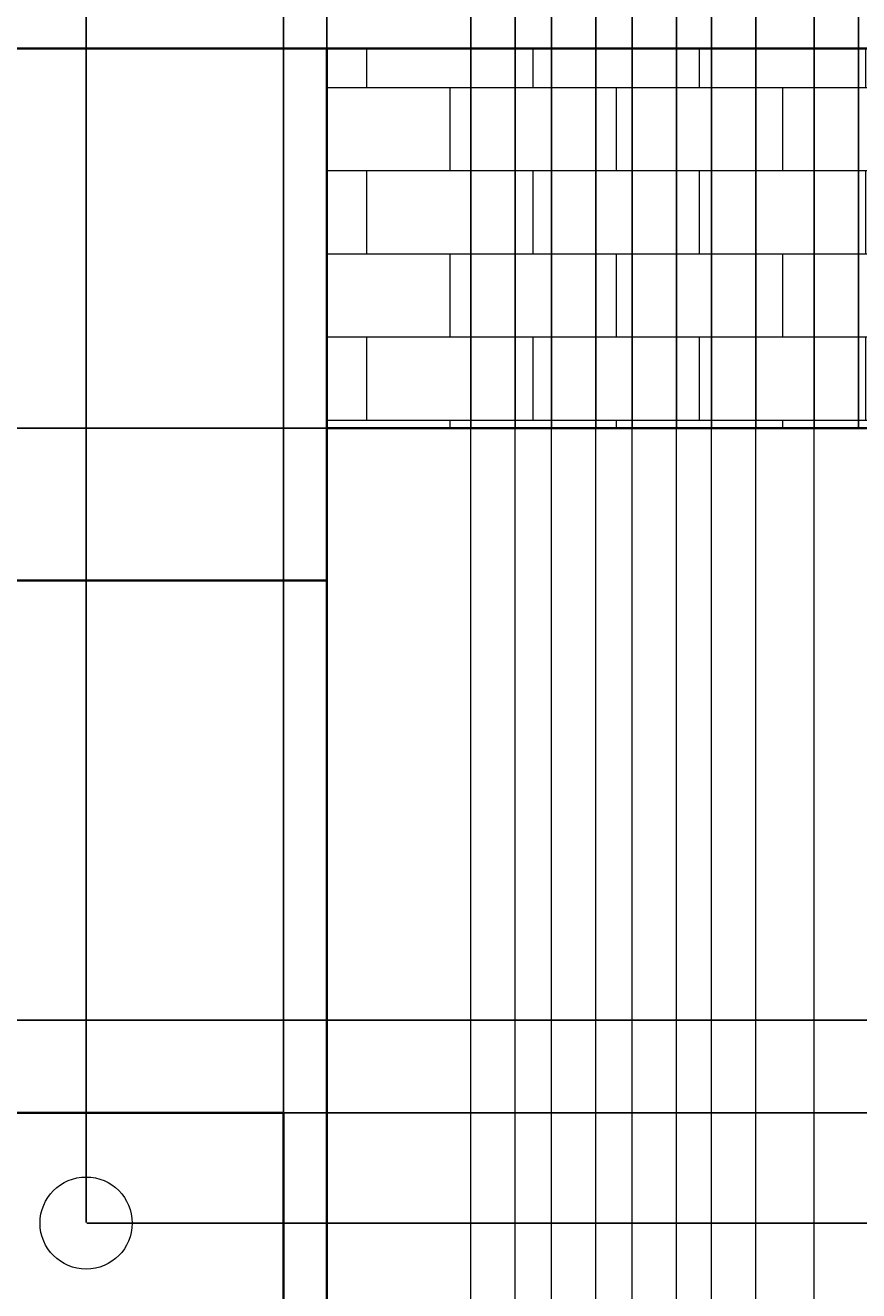
# Model space of a CAD drawing. Units: inches. Extents: x -13 to 809, y 112 to 656.
# Tile 34 of 55: x 314 to 389, y 446 to 561. Entities that reach past the tile are written whole.
import ezdxf

# ---------------------------------------------------------------- set-up
doc = ezdxf.new("R2010")
doc.units = ezdxf.units.IN
doc.header["$MEASUREMENT"] = 0
for name, color, linetype, lineweight in [('A-ANNO-DIMS', 2, 'Continuous', 18), ('A-ELEV', 7, 'Continuous', 35), ('A-ELEV-OTLN', 7, 'Continuous', 18), ('A-ELEV-PATT', 8, 'Continuous', 13)]:
    doc.layers.add(name, color=color, linetype=linetype, lineweight=lineweight)
doc.styles.get("Standard").update_dxf_attribs({"font": 'arial.ttf'})
doc.dimstyles.get("Standard").update_dxf_attribs({"dimtxt": 0.625, "dimasz": 0.18, "dimexe": 0.18, "dimexo": 0.0625, "dimgap": 0.09, "dimtad": 0, "dimtih": 1, "dimtoh": 1, "dimdec": 4, "dimzin": 0, "dimdsep": 46, "dimlunit": 4, "dimtxsty": 'Standard', "dimcen": 0.09, "dimadec": 0, "dimazin": 0, "dimtfac": 1, "dimtdec": 4, "dimtofl": 0, "dimtmove": 0, "dimatfit": 3, "dimfxl": 1, "dimtolj": 1, "dimtzin": 0, "dimarcsym": 0})

# ---------------------------------------------------------------- blocks, each defined once
blk = doc.blocks.new('*D25')
at = {"layer": 'A-ANNO-DIMS', "color": 0, "lineweight": -2, "transparency": 16777216}
for p, q in [((311.7, 617.43), (311.7, 655.96)), ((311.88, 655.78), (325.46, 655.78)), ((341.23, 655.78), (327.64, 655.78)), ((341.41, 524.34), (341.41, 655.96))]:
    blk.add_line(p, q, dxfattribs=at)
at = {"layer": 'A-ANNO-DIMS', "color": 0, "transparency": 16777216}
for points in [[(311.88, 655.81), (311.88, 655.75), (311.7, 655.78)], [(341.23, 655.81), (341.23, 655.75), (341.41, 655.78)]]:
    blk.add_solid(points, dxfattribs=at)
at = {"layer": 'Defpoints', "color": 0, "transparency": 16777216}
for p in [(341.41, 655.78), (311.7, 617.37), (341.41, 524.28)]:
    blk.add_point(p, dxfattribs=at)
at = {"layer": 'A-ANNO-DIMS', "color": 0, "transparency": 16777216, "insert": (326.55, 655.78), "char_height": 0.625, "attachment_point": 5}
blk.add_mtext('\\A1;29.71', dxfattribs=at)
blk = doc.blocks.new('*D26')
at = {"layer": 'A-ANNO-DIMS', "color": 0, "lineweight": -2, "transparency": 16777216}
for p, q in [((341.41, 524.34), (341.41, 655.96)), ((341.59, 655.78), (405.14, 655.78)), ((470.92, 655.78), (407.37, 655.78)), ((471.1, 470.94), (471.1, 655.96))]:
    blk.add_line(p, q, dxfattribs=at)
at = {"layer": 'A-ANNO-DIMS', "color": 0, "transparency": 16777216}
for points in [[(341.59, 655.81), (341.59, 655.75), (341.41, 655.78)], [(470.92, 655.81), (470.92, 655.75), (471.1, 655.78)]]:
    blk.add_solid(points, dxfattribs=at)
at = {"layer": 'Defpoints', "color": 0, "transparency": 16777216}
for p in [(471.1, 655.78), (341.41, 524.28), (471.1, 470.88)]:
    blk.add_point(p, dxfattribs=at)
at = {"layer": 'A-ANNO-DIMS', "color": 0, "transparency": 16777216, "insert": (406.25, 655.78), "char_height": 0.625, "attachment_point": 5}
blk.add_mtext('\\A1;129.7', dxfattribs=at)
blk = doc.blocks.new('*D39')
at = {"layer": 'A-ANNO-DIMS', "color": 0, "lineweight": -2, "transparency": 16777216}
for p, q in [((341.34, 524.28), (-12.1, 524.28)), ((-11.92, 524.1), (-11.92, 406.78)), ((-11.92, 288.63), (-11.92, 405.96)), ((341.34, 288.45), (-12.1, 288.45))]:
    blk.add_line(p, q, dxfattribs=at)
at = {"layer": 'A-ANNO-DIMS', "color": 0, "transparency": 16777216}
for points in [[(-11.95, 524.1), (-11.89, 524.1), (-11.92, 524.28)], [(-11.95, 288.63), (-11.89, 288.63), (-11.92, 288.45)]]:
    blk.add_solid(points, dxfattribs=at)
at = {"layer": 'Defpoints', "color": 0, "transparency": 16777216}
for p in [(-11.92, 524.28), (341.41, 524.28), (341.41, 288.45)]:
    blk.add_point(p, dxfattribs=at)
at = {"layer": 'A-ANNO-DIMS', "color": 0, "transparency": 16777216, "insert": (-11.92, 406.37), "char_height": 0.625, "attachment_point": 5}
blk.add_mtext('\\A1;235.83', dxfattribs=at)
blk = doc.blocks.new('*D43')
at = {"layer": 'A-ANNO-DIMS', "color": 0, "lineweight": -2, "transparency": 16777216}
for p, q in [((471.04, 470.88), (-12.1, 470.88)), ((-11.92, 470.7), (-11.92, 443.28)), ((-11.92, 415.04), (-11.92, 442.46)), ((471.04, 414.86), (-12.1, 414.86))]:
    blk.add_line(p, q, dxfattribs=at)
at = {"layer": 'A-ANNO-DIMS', "color": 0, "transparency": 16777216}
for points in [[(-11.95, 470.7), (-11.89, 470.7), (-11.92, 470.88)], [(-11.95, 415.04), (-11.89, 415.04), (-11.92, 414.86)]]:
    blk.add_solid(points, dxfattribs=at)
at = {"layer": 'Defpoints', "color": 0, "transparency": 16777216}
for p in [(-11.92, 470.88), (471.1, 470.88), (471.1, 414.86)]:
    blk.add_point(p, dxfattribs=at)
at = {"layer": 'A-ANNO-DIMS', "color": 0, "transparency": 16777216, "insert": (-11.92, 442.87), "char_height": 0.625, "attachment_point": 5}
blk.add_mtext('\\A1;56.02', dxfattribs=at)
blk = doc.blocks.new('*D53')
at = {"layer": 'A-ANNO-DIMS', "color": 0, "lineweight": -2, "transparency": 16777216}
for p, q in [((341.41, 524.34), (341.41, 655.96)), ((341.59, 655.78), (346.6, 655.78)), ((354.21, 655.78), (349.2, 655.78)), ((354.39, 524.34), (354.39, 655.96))]:
    blk.add_line(p, q, dxfattribs=at)
at = {"layer": 'A-ANNO-DIMS', "color": 0, "transparency": 16777216}
for points in [[(341.59, 655.81), (341.59, 655.75), (341.41, 655.78)], [(354.21, 655.81), (354.21, 655.75), (354.39, 655.78)]]:
    blk.add_solid(points, dxfattribs=at)
at = {"layer": 'Defpoints', "color": 0, "transparency": 16777216}
for p in [(354.39, 655.78), (341.41, 524.28), (354.39, 524.28)]:
    blk.add_point(p, dxfattribs=at)
at = {"layer": 'A-ANNO-DIMS', "color": 0, "transparency": 16777216, "insert": (347.9, 655.78), "char_height": 0.625, "attachment_point": 5}
blk.add_mtext('\\A1;12.981', dxfattribs=at)
blk = doc.blocks.new('*D54')
at = {"layer": 'A-ANNO-DIMS', "color": 0, "lineweight": -2, "transparency": 16777216}
for p, q in [((354.39, 524.34), (354.39, 655.96)), ((354.57, 655.78), (356.08, 655.78)), ((358.21, 655.78), (356.69, 655.78)), ((358.39, 524.34), (358.39, 655.96))]:
    blk.add_line(p, q, dxfattribs=at)
at = {"layer": 'A-ANNO-DIMS', "color": 0, "transparency": 16777216}
for points in [[(354.57, 655.81), (354.57, 655.75), (354.39, 655.78)], [(358.21, 655.81), (358.21, 655.75), (358.39, 655.78)]]:
    blk.add_solid(points, dxfattribs=at)
at = {"layer": 'Defpoints', "color": 0, "transparency": 16777216}
for p in [(358.39, 655.78), (354.39, 524.28), (358.39, 524.28)]:
    blk.add_point(p, dxfattribs=at)
at = {"layer": 'A-ANNO-DIMS', "color": 0, "transparency": 16777216, "insert": (356.39, 655.78), "char_height": 0.625, "attachment_point": 5}
blk.add_mtext('\\A1;4', dxfattribs=at)
blk = doc.blocks.new('*D55')
at = {"layer": 'A-ANNO-DIMS', "color": 0, "lineweight": -2, "transparency": 16777216}
for p, q in [((358.39, 524.34), (358.39, 655.96)), ((358.57, 655.78), (358.88, 655.78)), ((361.48, 655.78), (361.17, 655.78)), ((361.66, 524.34), (361.66, 655.96))]:
    blk.add_line(p, q, dxfattribs=at)
at = {"layer": 'A-ANNO-DIMS', "color": 0, "transparency": 16777216}
for points in [[(358.57, 655.81), (358.57, 655.75), (358.39, 655.78)], [(361.48, 655.81), (361.48, 655.75), (361.66, 655.78)]]:
    blk.add_solid(points, dxfattribs=at)
at = {"layer": 'Defpoints', "color": 0, "transparency": 16777216}
for p in [(361.66, 655.78), (358.39, 524.28), (361.66, 524.28)]:
    blk.add_point(p, dxfattribs=at)
at = {"layer": 'A-ANNO-DIMS', "color": 0, "transparency": 16777216, "insert": (360.03, 655.78), "char_height": 0.625, "attachment_point": 5}
blk.add_mtext('\\A1;3.274', dxfattribs=at)
blk = doc.blocks.new('*D56')
at = {"layer": 'A-ANNO-DIMS', "color": 0, "lineweight": -2, "transparency": 16777216}
for p, q in [((361.66, 524.34), (361.66, 655.96)), ((361.84, 655.78), (363.36, 655.78)), ((365.48, 655.78), (363.97, 655.78)), ((365.66, 524.34), (365.66, 655.96))]:
    blk.add_line(p, q, dxfattribs=at)
at = {"layer": 'A-ANNO-DIMS', "color": 0, "transparency": 16777216}
for points in [[(361.84, 655.81), (361.84, 655.75), (361.66, 655.78)], [(365.48, 655.81), (365.48, 655.75), (365.66, 655.78)]]:
    blk.add_solid(points, dxfattribs=at)
at = {"layer": 'Defpoints', "color": 0, "transparency": 16777216}
for p in [(365.66, 655.78), (361.66, 524.28), (365.66, 524.28)]:
    blk.add_point(p, dxfattribs=at)
at = {"layer": 'A-ANNO-DIMS', "color": 0, "transparency": 16777216, "insert": (363.66, 655.78), "char_height": 0.625, "attachment_point": 5}
blk.add_mtext('\\A1;4', dxfattribs=at)
blk = doc.blocks.new('*D57')
at = {"layer": 'A-ANNO-DIMS', "color": 0, "lineweight": -2, "transparency": 16777216}
for p, q in [((365.66, 524.34), (365.66, 655.96)), ((365.84, 655.78), (366.15, 655.78)), ((368.74, 655.78), (368.44, 655.78)), ((368.92, 524.34), (368.92, 655.96))]:
    blk.add_line(p, q, dxfattribs=at)
at = {"layer": 'A-ANNO-DIMS', "color": 0, "transparency": 16777216}
for points in [[(365.84, 655.81), (365.84, 655.75), (365.66, 655.78)], [(368.74, 655.81), (368.74, 655.75), (368.92, 655.78)]]:
    blk.add_solid(points, dxfattribs=at)
at = {"layer": 'Defpoints', "color": 0, "transparency": 16777216}
for p in [(368.92, 655.78), (365.66, 524.28), (368.92, 524.28)]:
    blk.add_point(p, dxfattribs=at)
at = {"layer": 'A-ANNO-DIMS', "color": 0, "transparency": 16777216, "insert": (367.29, 655.78), "char_height": 0.625, "attachment_point": 5}
blk.add_mtext('\\A1;3.259', dxfattribs=at)
blk = doc.blocks.new('*D58')
at = {"layer": 'A-ANNO-DIMS', "color": 0, "lineweight": -2, "transparency": 16777216}
for p, q in [((368.92, 524.34), (368.92, 655.96)), ((369.1, 655.78), (370.62, 655.78)), ((372.74, 655.78), (371.23, 655.78)), ((372.92, 524.34), (372.92, 655.96))]:
    blk.add_line(p, q, dxfattribs=at)
at = {"layer": 'A-ANNO-DIMS', "color": 0, "transparency": 16777216}
for points in [[(369.1, 655.81), (369.1, 655.75), (368.92, 655.78)], [(372.74, 655.81), (372.74, 655.75), (372.92, 655.78)]]:
    blk.add_solid(points, dxfattribs=at)
at = {"layer": 'Defpoints', "color": 0, "transparency": 16777216}
for p in [(372.92, 655.78), (368.92, 524.28), (372.92, 524.28)]:
    blk.add_point(p, dxfattribs=at)
at = {"layer": 'A-ANNO-DIMS', "color": 0, "transparency": 16777216, "insert": (370.92, 655.78), "char_height": 0.625, "attachment_point": 5}
blk.add_mtext('\\A1;4', dxfattribs=at)
blk = doc.blocks.new('*D59')
at = {"layer": 'A-ANNO-DIMS', "color": 0, "lineweight": -2, "transparency": 16777216}
for p, q in [((372.92, 524.34), (372.92, 655.96)), ((373.1, 655.78), (373.36, 655.78)), ((375.91, 655.78), (375.65, 655.78)), ((376.09, 524.34), (376.09, 655.96))]:
    blk.add_line(p, q, dxfattribs=at)
at = {"layer": 'A-ANNO-DIMS', "color": 0, "transparency": 16777216}
for points in [[(373.1, 655.81), (373.1, 655.75), (372.92, 655.78)], [(375.91, 655.81), (375.91, 655.75), (376.09, 655.78)]]:
    blk.add_solid(points, dxfattribs=at)
at = {"layer": 'Defpoints', "color": 0, "transparency": 16777216}
for p in [(376.09, 655.78), (372.92, 524.28), (376.09, 524.28)]:
    blk.add_point(p, dxfattribs=at)
at = {"layer": 'A-ANNO-DIMS', "color": 0, "transparency": 16777216, "insert": (374.5, 655.78), "char_height": 0.625, "attachment_point": 5}
blk.add_mtext('\\A1;3.165', dxfattribs=at)
blk = doc.blocks.new('*D60')
at = {"layer": 'A-ANNO-DIMS', "color": 0, "lineweight": -2, "transparency": 16777216}
for p, q in [((376.09, 524.34), (376.09, 655.96)), ((376.27, 655.78), (377.78, 655.78)), ((379.91, 655.78), (378.39, 655.78)), ((380.09, 524.34), (380.09, 655.96))]:
    blk.add_line(p, q, dxfattribs=at)
at = {"layer": 'A-ANNO-DIMS', "color": 0, "transparency": 16777216}
for points in [[(376.27, 655.81), (376.27, 655.75), (376.09, 655.78)], [(379.91, 655.81), (379.91, 655.75), (380.09, 655.78)]]:
    blk.add_solid(points, dxfattribs=at)
at = {"layer": 'Defpoints', "color": 0, "transparency": 16777216}
for p in [(380.09, 655.78), (376.09, 524.28), (380.09, 524.28)]:
    blk.add_point(p, dxfattribs=at)
at = {"layer": 'A-ANNO-DIMS', "color": 0, "transparency": 16777216, "insert": (378.09, 655.78), "char_height": 0.625, "attachment_point": 5}
blk.add_mtext('\\A1;4', dxfattribs=at)
blk = doc.blocks.new('*D61')
at = {"layer": 'A-ANNO-DIMS', "color": 0, "lineweight": -2, "transparency": 16777216}
for p, q in [((380.09, 524.34), (380.09, 655.96)), ((380.27, 655.78), (381.58, 655.78)), ((385.17, 655.78), (383.86, 655.78)), ((385.35, 524.34), (385.35, 655.96))]:
    blk.add_line(p, q, dxfattribs=at)
at = {"layer": 'A-ANNO-DIMS', "color": 0, "transparency": 16777216}
for points in [[(380.27, 655.81), (380.27, 655.75), (380.09, 655.78)], [(385.17, 655.81), (385.17, 655.75), (385.35, 655.78)]]:
    blk.add_solid(points, dxfattribs=at)
at = {"layer": 'Defpoints', "color": 0, "transparency": 16777216}
for p in [(385.35, 655.78), (380.09, 524.28), (385.35, 524.28)]:
    blk.add_point(p, dxfattribs=at)
at = {"layer": 'A-ANNO-DIMS', "color": 0, "transparency": 16777216, "insert": (382.72, 655.78), "char_height": 0.625, "attachment_point": 5}
blk.add_mtext('\\A1;5.267', dxfattribs=at)
blk = doc.blocks.new('*D62')
at = {"layer": 'A-ANNO-DIMS', "color": 0, "lineweight": -2, "transparency": 16777216}
for p, q in [((385.35, 524.34), (385.35, 655.96)), ((385.53, 655.78), (387.05, 655.78)), ((389.17, 655.78), (387.66, 655.78)), ((389.35, 524.34), (389.35, 655.96))]:
    blk.add_line(p, q, dxfattribs=at)
at = {"layer": 'A-ANNO-DIMS', "color": 0, "transparency": 16777216}
for points in [[(385.53, 655.81), (385.53, 655.75), (385.35, 655.78)], [(389.17, 655.81), (389.17, 655.75), (389.35, 655.78)]]:
    blk.add_solid(points, dxfattribs=at)
at = {"layer": 'Defpoints', "color": 0, "transparency": 16777216}
for p in [(389.35, 655.78), (385.35, 524.28), (389.35, 524.28)]:
    blk.add_point(p, dxfattribs=at)
at = {"layer": 'A-ANNO-DIMS', "color": 0, "transparency": 16777216, "insert": (387.35, 655.78), "char_height": 0.625, "attachment_point": 5}
blk.add_mtext('\\A1;4', dxfattribs=at)
blk = doc.blocks.new('*D63')
at = {"layer": 'A-ANNO-DIMS', "color": 0, "lineweight": -2, "transparency": 16777216}
for p, q in [((389.35, 524.34), (389.35, 655.96)), ((389.53, 655.78), (389.69, 655.78)), ((392.15, 655.78), (391.99, 655.78)), ((392.33, 524.34), (392.33, 655.96))]:
    blk.add_line(p, q, dxfattribs=at)
at = {"layer": 'A-ANNO-DIMS', "color": 0, "transparency": 16777216}
for points in [[(389.53, 655.81), (389.53, 655.75), (389.35, 655.78)], [(392.15, 655.81), (392.15, 655.75), (392.33, 655.78)]]:
    blk.add_solid(points, dxfattribs=at)
at = {"layer": 'Defpoints', "color": 0, "transparency": 16777216}
for p in [(392.33, 655.78), (389.35, 524.28), (392.33, 524.28)]:
    blk.add_point(p, dxfattribs=at)
at = {"layer": 'A-ANNO-DIMS', "color": 0, "transparency": 16777216, "insert": (390.84, 655.78), "char_height": 0.625, "attachment_point": 5}
blk.add_mtext('\\A1;2.974', dxfattribs=at)
blk = doc.blocks.new('*D102')
at = {"layer": 'A-ANNO-DIMS', "color": 0, "lineweight": -2, "transparency": 16777216}
for p, q in [((292.68, 452.63), (292.68, 655.96)), ((292.86, 655.78), (304.8, 655.78)), ((319.52, 655.78), (307.58, 655.78)), ((319.7, 452.63), (319.7, 655.96))]:
    blk.add_line(p, q, dxfattribs=at)
at = {"layer": 'A-ANNO-DIMS', "color": 0, "transparency": 16777216}
for points in [[(292.86, 655.81), (292.86, 655.75), (292.68, 655.78)], [(319.52, 655.81), (319.52, 655.75), (319.7, 655.78)]]:
    blk.add_solid(points, dxfattribs=at)
at = {"layer": 'Defpoints', "color": 0, "transparency": 16777216}
for p in [(319.7, 655.78), (292.68, 452.56), (319.7, 452.56)]:
    blk.add_point(p, dxfattribs=at)
at = {"layer": 'A-ANNO-DIMS', "color": 0, "transparency": 16777216, "insert": (306.19, 655.78), "char_height": 0.625, "attachment_point": 5}
blk.add_mtext('\\A1;27.017', dxfattribs=at)
blk = doc.blocks.new('*D103')
at = {"layer": 'A-ANNO-DIMS', "color": 0, "lineweight": -2, "transparency": 16777216}
for p, q in [((319.7, 452.63), (319.7, 655.96)), ((319.88, 655.78), (327.25, 655.78)), ((337.33, 655.78), (329.96, 655.78)), ((337.51, 462.58), (337.51, 655.96))]:
    blk.add_line(p, q, dxfattribs=at)
at = {"layer": 'A-ANNO-DIMS', "color": 0, "transparency": 16777216}
for points in [[(319.88, 655.81), (319.88, 655.75), (319.7, 655.78)], [(337.33, 655.81), (337.33, 655.75), (337.51, 655.78)]]:
    blk.add_solid(points, dxfattribs=at)
at = {"layer": 'Defpoints', "color": 0, "transparency": 16777216}
for p in [(337.51, 655.78), (337.51, 462.52), (319.7, 452.56)]:
    blk.add_point(p, dxfattribs=at)
at = {"layer": 'A-ANNO-DIMS', "color": 0, "transparency": 16777216, "insert": (328.6, 655.78), "char_height": 0.625, "attachment_point": 5}
blk.add_mtext('\\A1;17.807', dxfattribs=at)
blk = doc.blocks.new('*D104')
at = {"layer": 'A-ANNO-DIMS', "color": 0, "lineweight": -2, "transparency": 16777216}
for p, q in [((337.57, 462.52), (807.77, 462.52)), ((807.59, 462.34), (807.59, 457.95)), ((807.59, 452.74), (807.59, 457.13)), ((319.76, 452.56), (807.77, 452.56))]:
    blk.add_line(p, q, dxfattribs=at)
at = {"layer": 'A-ANNO-DIMS', "color": 0, "transparency": 16777216}
for points in [[(807.56, 462.34), (807.62, 462.34), (807.59, 462.52)], [(807.56, 452.74), (807.62, 452.74), (807.59, 452.56)]]:
    blk.add_solid(points, dxfattribs=at)
at = {"layer": 'Defpoints', "color": 0, "transparency": 16777216}
for p in [(337.51, 462.52), (319.7, 452.56), (807.59, 452.56)]:
    blk.add_point(p, dxfattribs=at)
at = {"layer": 'A-ANNO-DIMS', "color": 0, "transparency": 16777216, "insert": (807.59, 457.54), "char_height": 0.625, "attachment_point": 5}
blk.add_mtext('\\A1;9.957', dxfattribs=at)
blk = doc.blocks.new('*D105')
at = {"layer": 'A-ANNO-DIMS', "color": 0, "lineweight": -2, "transparency": 16777216}
for p, q in [((319.76, 452.56), (807.77, 452.56)), ((807.59, 452.38), (807.59, 448.95)), ((807.59, 444.7), (807.59, 448.13)), ((319.57, 444.52), (807.77, 444.52))]:
    blk.add_line(p, q, dxfattribs=at)
at = {"layer": 'A-ANNO-DIMS', "color": 0, "transparency": 16777216}
for points in [[(807.56, 452.38), (807.62, 452.38), (807.59, 452.56)], [(807.56, 444.7), (807.62, 444.7), (807.59, 444.52)]]:
    blk.add_solid(points, dxfattribs=at)
at = {"layer": 'Defpoints', "color": 0, "transparency": 16777216}
for p in [(319.7, 452.56), (319.51, 444.52), (807.59, 444.52)]:
    blk.add_point(p, dxfattribs=at)
at = {"layer": 'A-ANNO-DIMS', "color": 0, "transparency": 16777216, "insert": (807.59, 448.54), "char_height": 0.625, "attachment_point": 5}
blk.add_mtext('\\A1;8.043', dxfattribs=at)

msp = doc.modelspace()

# ---------------------------------------------------------------- hatches: boundary and pattern name
at = {"layer": 'A-ELEV-PATT'}
h = msp.add_hatch(dxfattribs=at)
h.set_pattern_fill('BRICK', color=256, scale=30)
h.paths.add_polyline_path([(591.008, 558.5199), (341.4072, 558.5199), (341.4072, 524.281), (542.9617, 524.281), (542.9617, 288.4508), (341.4072, 288.4508), (341.4072, 250.8429), (591.008, 250.8429)])

# ---------------------------------------------------------------- linework, layer by layer
at = {"layer": 'A-ELEV'}
for p, q in [((341.4072, 558.5199), (292.923, 558.5199)), ((341.4072, 524.281), (341.4072, 558.5199)), ((341.4072, 510.5199), (341.4072, 558.5199)), ((341.4072, 558.5199), (591.008, 558.5199)), ((341.4072, 210.7849), (341.4072, 524.281)), ((107.2588, 510.5199), (341.4072, 510.5199)), ((95.0469, 462.5199), (337.5074, 462.5199)), ((337.5074, 462.5199), (337.5074, 306.5199))]:
    msp.add_line(p, q, dxfattribs=at)
for points in [[(341.4072, 558.5199), (591.008, 558.5199), (591.008, 250.8429), (341.4072, 250.8429)], [(341.4072, 524.281), (542.9617, 524.281), (542.9617, 288.4508), (341.4072, 288.4508)]]:
    msp.add_lwpolyline(points, close=True, dxfattribs=at)
at = {"layer": 'A-ELEV-OTLN'}
msp.add_circle((319.7004, 452.5629), 4.1542, dxfattribs=at)
at = {"layer": 'A-ELEV-PATT'}
for points in [[(354.3886, 288.4508), (354.3886, 523.3908), (354.3886, 524.281)], [(358.3886, 288.4508), (358.3886, 523.3908), (358.3886, 524.281)], [(361.6625, 288.4508), (361.6625, 523.3908), (361.6625, 524.281)], [(365.6625, 288.4508), (365.6625, 523.3908), (365.6625, 524.281)], [(368.9215, 288.4508), (368.9215, 523.3908), (368.9215, 524.281)], [(372.9215, 288.4508), (372.9215, 523.3908), (372.9215, 524.281)], [(376.0866, 288.4508), (376.0866, 523.3908), (376.0866, 524.281)], [(380.0866, 288.4508), (380.0866, 523.3908), (380.0866, 524.281)], [(385.3536, 288.4508), (385.3536, 523.3908), (385.3536, 524.281)]]:
    msp.add_lwpolyline(points, dxfattribs=at)

# ---------------------------------------------------------------- dimensions: what is measured, and where the dimension line sits
at = {"layer": 'A-ANNO-DIMS'}
for base, p1, p2, override, picture, middle in [((319.7004, 655.7828), (292.6832, 452.5629), (319.7004, 452.5629), {"dimdec": 3, "dimlfac": 1, "dimrnd": 0, "dimzin": 0, "dimdsep": 46, "dimlunit": 2}, '*D102', (306.1918, 655.7828)), ((341.4072, 655.7828), (311.6991, 617.3708), (341.4072, 524.281), {"dimdec": 2, "dimlfac": 1, "dimrnd": 0, "dimzin": 0, "dimdsep": 46, "dimlunit": 2}, '*D25', (326.5531, 655.7828)), ((337.5074, 655.7828), (319.7004, 452.5629), (337.5074, 462.5199), {"dimdec": 3, "dimlfac": 1, "dimrnd": 0, "dimzin": 0, "dimdsep": 46, "dimlunit": 2}, '*D103', (328.6039, 655.7828)), ((471.0998, 655.7828), (341.4072, 524.281), (471.0998, 470.8765), {"dimdec": 1, "dimlfac": 1, "dimrnd": 0, "dimzin": 0, "dimdsep": 46, "dimlunit": 2}, '*D26', (406.2535, 655.7828)), ((354.3886, 655.7828), (341.4072, 524.281), (354.3886, 524.281), {"dimdec": 3, "dimlfac": 1, "dimrnd": 0, "dimzin": 0, "dimdsep": 46, "dimlunit": 2}, '*D53', (347.8979, 655.7828)), ((358.3886, 655.7828), (354.3886, 524.281), (358.3886, 524.281), {"dimdec": 0, "dimlfac": 1, "dimrnd": 0, "dimzin": 0, "dimdsep": 46, "dimlunit": 2}, '*D54', (356.3886, 655.7828)), ((361.6625, 655.7828), (358.3886, 524.281), (361.6625, 524.281), {"dimdec": 3, "dimlfac": 1, "dimrnd": 0, "dimzin": 0, "dimdsep": 46, "dimlunit": 2}, '*D55', (360.0256, 655.7828)), ((365.6625, 655.7828), (361.6625, 524.281), (365.6625, 524.281), {"dimdec": 0, "dimlfac": 1, "dimrnd": 0, "dimzin": 0, "dimdsep": 46, "dimlunit": 2}, '*D56', (363.6625, 655.7828)), ((368.9215, 655.7828), (365.6625, 524.281), (368.9215, 524.281), {"dimdec": 3, "dimlfac": 1, "dimrnd": 0, "dimzin": 0, "dimdsep": 46, "dimlunit": 2}, '*D57', (367.292, 655.7828)), ((372.9215, 655.7828), (368.9215, 524.281), (372.9215, 524.281), {"dimdec": 0, "dimlfac": 1, "dimrnd": 0, "dimzin": 0, "dimdsep": 46, "dimlunit": 2}, '*D58', (370.9215, 655.7828)), ((376.0866, 655.7828), (372.9215, 524.281), (376.0866, 524.281), {"dimdec": 3, "dimlfac": 1, "dimrnd": 0, "dimzin": 0, "dimdsep": 46, "dimlunit": 2}, '*D59', (374.504, 655.7828)), ((380.0866, 655.7828), (376.0866, 524.281), (380.0866, 524.281), {"dimdec": 0, "dimlfac": 1, "dimrnd": 0, "dimzin": 0, "dimdsep": 46, "dimlunit": 2}, '*D60', (378.0866, 655.7828)), ((385.3536, 655.7828), (380.0866, 524.281), (385.3536, 524.281), {"dimdec": 3, "dimlfac": 1, "dimrnd": 0, "dimzin": 0, "dimdsep": 46, "dimlunit": 2}, '*D61', (382.7201, 655.7828)), ((389.3536, 655.7828), (385.3536, 524.281), (389.3536, 524.281), {"dimdec": 0, "dimlfac": 1, "dimrnd": 0, "dimzin": 0, "dimdsep": 46, "dimlunit": 2}, '*D62', (387.3536, 655.7828)), ((392.3277, 655.7828), (389.3536, 524.281), (392.3277, 524.281), {"dimdec": 3, "dimlfac": 1, "dimrnd": 0, "dimzin": 0, "dimdsep": 46, "dimlunit": 2}, '*D63', (390.8407, 655.7828))]:
    dim = msp.add_linear_dim(base=base, p1=p1, p2=p2, dimstyle='Standard', override=override, dxfattribs=at)
    dim.commit()
    dim.dimension.update_dxf_attribs({"geometry": picture, "text_midpoint": middle})
for base, p1, p2, override, picture, middle in [((-11.9191, 524.281), (341.4072, 288.4508), (341.4072, 524.281), {"dimdec": 2, "dimlfac": 1, "dimrnd": 0, "dimzin": 0, "dimdsep": 46, "dimlunit": 2}, '*D39', (-11.9191, 406.3659)), ((-11.9191, 470.8765), (471.0998, 414.8594), (471.0998, 470.8765), {"dimdec": 2, "dimlfac": 1, "dimrnd": 0, "dimzin": 0, "dimdsep": 46, "dimlunit": 2}, '*D43', (-11.9191, 442.8679)), ((807.5888, 452.5629), (337.5074, 462.5199), (319.7004, 452.5629), {"dimdec": 3, "dimlfac": 1, "dimrnd": 0, "dimzin": 0, "dimdsep": 46, "dimlunit": 2}, '*D104', (807.5888, 457.5414)), ((807.5888, 444.5199), (319.7004, 452.5629), (319.5074, 444.5199), {"dimdec": 3, "dimlfac": 1, "dimrnd": 0, "dimzin": 0, "dimdsep": 46, "dimlunit": 2}, '*D105', (807.5888, 448.5414))]:
    dim = msp.add_linear_dim(base=base, p1=p1, p2=p2, angle=90, dimstyle='Standard', override=override, dxfattribs=at)
    dim.commit()
    dim.dimension.update_dxf_attribs({"geometry": picture, "text_midpoint": middle})

doc.saveas('drawing.dxf')
